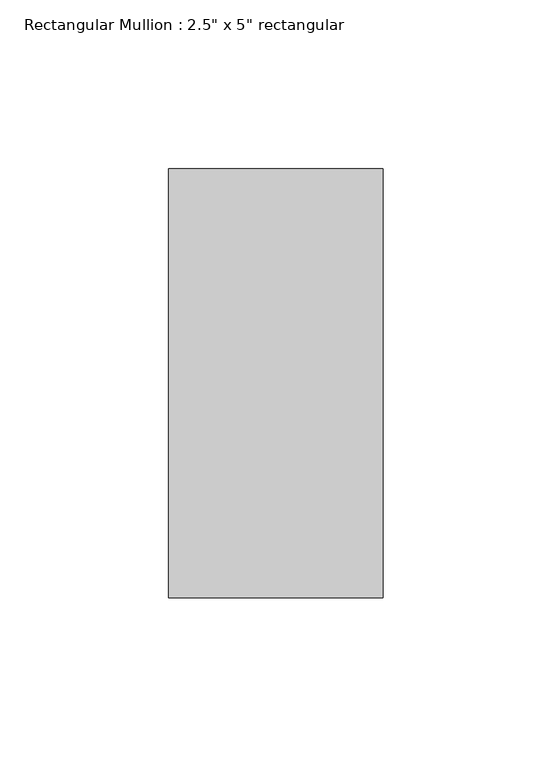
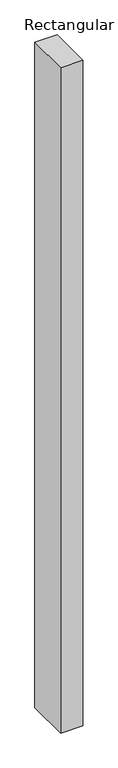
"""IFC4 building model written with IfcOpenShell, lengths in millimetres: member geometry."""

from ifc_helpers import new_model, si_unit, frame, origin, place, context, project, spatial, polyline, outline, extrude, source, transform, mapped, element, save


def member_16b81337(model_context):
    return source(origin(), model_context, "Body", "SweptSolid", [
        extrude(outline(polyline([(0.0, 63.5), (0.0, -63.5), (-63.5, -63.5), (-63.5, 63.5), (0.0, 63.5)])), frame((0.0, 0.0, -2006.6), z_axis=(0.0, 0.0, 1.0), x_axis=(1.0, 0.0, 0.0)), (0.0, 0.0, 1.0), 2006.6),
    ])


if __name__ == "__main__":
    model = new_model("IFC4")
    model_context = context("Model", 3, world=origin())
    ifc_project = project(units=[si_unit("LENGTHUNIT", "METRE", prefix="MILLI")], contexts=[model_context])
    site = spatial("IfcSite", under=ifc_project)
    building = spatial("IfcBuilding", under=site)
    placement = place(None, origin())
    member_shape = member_16b81337(model_context)
    element("IfcMember", 1, ObjectType="Rectangular Mullion : 2.5\" x 5\" rectangular", at=placement, inside=building, context=model_context, shape_type="MappedRepresentation", body=[
        mapped(member_shape, transform((0.0, 0.0, 0.0), x_axis=(1.0, 0.0, 0.0), y_axis=(0.0, 1.0, 0.0), z_axis=(0.0, 0.0, 1.0))),
    ])
    save(model, "model.ifc")

# Revit data of these elements
# Type "Rectangular Mullion : 2.5\" x 5\" rectangular"
#   built-in parameter 1007304 = 0.416667 (stored number, unit not read)
#   built-in parameter 1007301 = 0.104167 (stored number, unit not read)
#   built-in parameter 1007300 = 0.104167 (stored number, unit not read)
# Element 1 (IfcMember, "Rectangular Mullion : 2.5\" x 5\" rectangular")
#   Materials on its faces: "door black"
# Materials
#   "door black": class "Generic", colour RGB 120 120 120, transparency 0, Cost = 0
